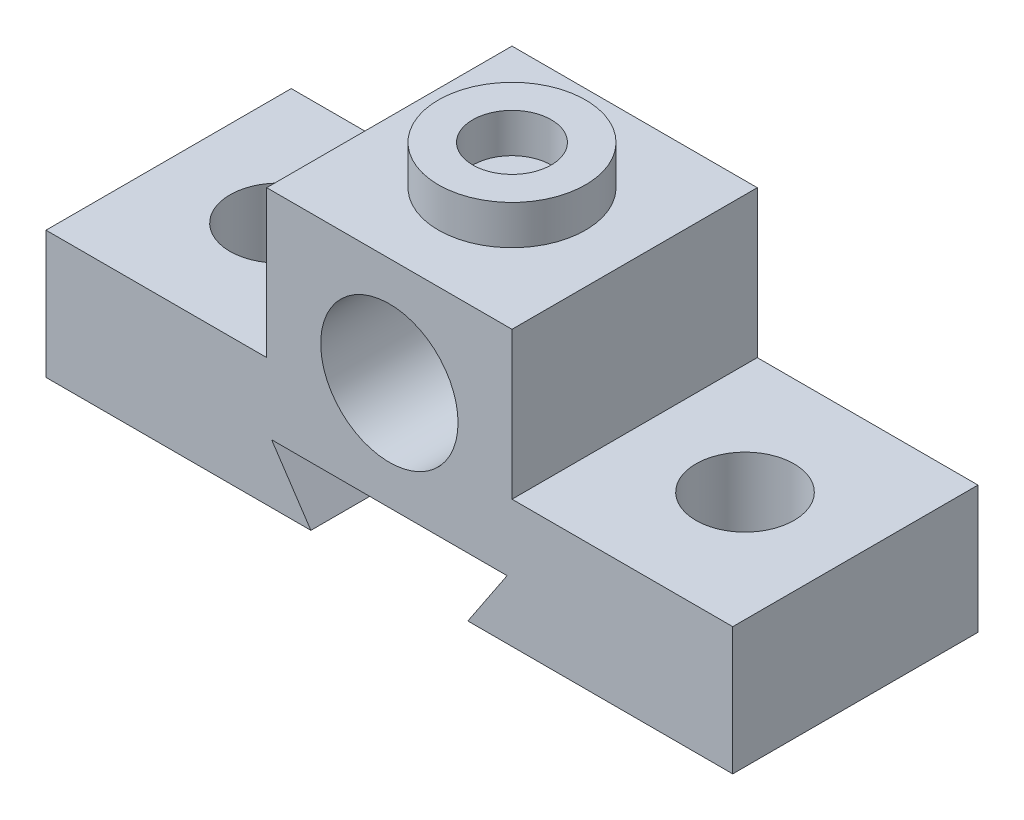
ISO-10303-21;
HEADER;
FILE_DESCRIPTION(('STEP AP214'),'2;1');
FILE_NAME('part.step','',(''),(''),'','','');
FILE_SCHEMA(('AUTOMOTIVE_DESIGN { 1 0 10303 214 1 1 1 1 }'));
ENDSEC;
DATA;
#1=APPLICATION_CONTEXT('core data for automotive mechanical design processes');
#2=APPLICATION_PROTOCOL_DEFINITION('international standard','automotive_design',2000,#1);
#3=PRODUCT_CONTEXT('',#1,'mechanical');
#4=PRODUCT('Part','Part','',(#3));
#5=PRODUCT_RELATED_PRODUCT_CATEGORY('part','',(#4));
#6=PRODUCT_DEFINITION_FORMATION('','',#4);
#7=PRODUCT_DEFINITION_CONTEXT('part definition',#1,'design');
#8=PRODUCT_DEFINITION('design','',#6,#7);
#9=PRODUCT_DEFINITION_SHAPE('','',#8);
#10=(LENGTH_UNIT() NAMED_UNIT(*) SI_UNIT(.MILLI.,.METRE.));
#11=(NAMED_UNIT(*) PLANE_ANGLE_UNIT() SI_UNIT($,.RADIAN.));
#12=(NAMED_UNIT(*) SI_UNIT($,.STERADIAN.) SOLID_ANGLE_UNIT());
#13=UNCERTAINTY_MEASURE_WITH_UNIT(LENGTH_MEASURE(1.E-05),#10,'distance_accuracy_value','');
#14=(GEOMETRIC_REPRESENTATION_CONTEXT(3) GLOBAL_UNCERTAINTY_ASSIGNED_CONTEXT((#13)) GLOBAL_UNIT_ASSIGNED_CONTEXT((#10,
#11,#12)) REPRESENTATION_CONTEXT('',''));
#15=CARTESIAN_POINT('',(0.,0.,0.));
#16=DIRECTION('',(0.,0.,1.));
#17=DIRECTION('',(1.,0.,0.));
#18=AXIS2_PLACEMENT_3D('',#15,#16,#17);
#19=CARTESIAN_POINT('',(0.,0.,25.));
#20=DIRECTION('',(0.,1.,0.));
#21=DIRECTION('',(0.,0.,1.));
#22=AXIS2_PLACEMENT_3D('',#19,#20,#21);
#23=PLANE('',#22);
#24=CARTESIAN_POINT('',(11.25,0.,12.5));
#25=DIRECTION('',(0.,1.,0.));
#26=DIRECTION('',(0.,0.,1.));
#27=AXIS2_PLACEMENT_3D('',#24,#25,#26);
#28=CIRCLE('',#27,5.);
#29=CARTESIAN_POINT('',(11.25,0.,17.5));
#30=VERTEX_POINT('',#29);
#31=EDGE_CURVE('E285',#30,#30,#28,.T.);
#32=ORIENTED_EDGE('',*,*,#31,.T.);
#33=EDGE_LOOP('',(#32));
#34=FACE_BOUND('',#33,.T.);
#35=DIRECTION('',(1.,0.,0.));
#36=VECTOR('',#35,1.);
#37=CARTESIAN_POINT('',(0.,0.,0.));
#38=LINE('',#37,#36);
#39=CARTESIAN_POINT('',(0.,0.,0.));
#40=VERTEX_POINT('',#39);
#41=CARTESIAN_POINT('',(27.,0.,0.));
#42=VERTEX_POINT('',#41);
#43=EDGE_CURVE('E170',#40,#42,#38,.T.);
#44=ORIENTED_EDGE('',*,*,#43,.T.);
#45=DIRECTION('',(0.,0.,-1.));
#46=VECTOR('',#45,1.);
#47=CARTESIAN_POINT('',(27.,0.,25.));
#48=LINE('',#47,#46);
#49=CARTESIAN_POINT('',(27.,0.,25.));
#50=VERTEX_POINT('',#49);
#51=EDGE_CURVE('E48',#50,#42,#48,.T.);
#52=ORIENTED_EDGE('',*,*,#51,.F.);
#53=DIRECTION('',(1.,0.,0.));
#54=VECTOR('',#53,1.);
#55=CARTESIAN_POINT('',(0.,0.,25.));
#56=LINE('',#55,#54);
#57=CARTESIAN_POINT('',(0.,0.,25.));
#58=VERTEX_POINT('',#57);
#59=EDGE_CURVE('E195',#58,#50,#56,.T.);
#60=ORIENTED_EDGE('',*,*,#59,.F.);
#61=DIRECTION('',(0.,0.,-1.));
#62=VECTOR('',#61,1.);
#63=CARTESIAN_POINT('',(0.,0.,25.));
#64=LINE('',#63,#62);
#65=EDGE_CURVE('E162',#58,#40,#64,.T.);
#66=ORIENTED_EDGE('',*,*,#65,.T.);
#67=EDGE_LOOP('',(#44,#52,#60,#66));
#68=FACE_BOUND('',#67,.T.);
#69=ADVANCED_FACE('F44',(#34,#68),#23,.F.);
#70=CARTESIAN_POINT('',(27.,0.,25.));
#71=DIRECTION('',(-0.832050294337844,-0.554700196225229,0.));
#72=DIRECTION('',(0.554700196225229,-0.832050294337844,0.));
#73=AXIS2_PLACEMENT_3D('',#70,#71,#72);
#74=PLANE('',#73);
#75=DIRECTION('',(-0.554700196225229,0.832050294337844,0.));
#76=VECTOR('',#75,1.);
#77=CARTESIAN_POINT('',(27.,0.,0.));
#78=LINE('',#77,#76);
#79=CARTESIAN_POINT('',(23.,6.,0.));
#80=VERTEX_POINT('',#79);
#81=EDGE_CURVE('E168',#42,#80,#78,.T.);
#82=ORIENTED_EDGE('',*,*,#81,.T.);
#83=DIRECTION('',(0.,0.,-1.));
#84=VECTOR('',#83,1.);
#85=CARTESIAN_POINT('',(23.,6.,25.));
#86=LINE('',#85,#84);
#87=CARTESIAN_POINT('',(23.,6.,25.));
#88=VERTEX_POINT('',#87);
#89=EDGE_CURVE('E213',#88,#80,#86,.T.);
#90=ORIENTED_EDGE('',*,*,#89,.F.);
#91=DIRECTION('',(-0.554700196225229,0.832050294337844,0.));
#92=VECTOR('',#91,1.);
#93=CARTESIAN_POINT('',(27.,0.,25.));
#94=LINE('',#93,#92);
#95=EDGE_CURVE('E120',#50,#88,#94,.T.);
#96=ORIENTED_EDGE('',*,*,#95,.F.);
#97=ORIENTED_EDGE('',*,*,#51,.T.);
#98=EDGE_LOOP('',(#82,#90,#96,#97));
#99=FACE_BOUND('',#98,.T.);
#100=ADVANCED_FACE('F217',(#99),#74,.F.);
#101=CARTESIAN_POINT('',(35.,6.,25.));
#102=DIRECTION('',(0.,1.,0.));
#103=DIRECTION('',(0.,0.,1.));
#104=AXIS2_PLACEMENT_3D('',#101,#102,#103);
#105=PLANE('',#104);
#106=DIRECTION('',(1.,0.,0.));
#107=VECTOR('',#106,1.);
#108=CARTESIAN_POINT('',(35.,6.,0.));
#109=LINE('',#108,#107);
#110=CARTESIAN_POINT('',(47.,6.,0.));
#111=VERTEX_POINT('',#110);
#112=EDGE_CURVE('E171',#80,#111,#109,.T.);
#113=ORIENTED_EDGE('',*,*,#112,.T.);
#114=DIRECTION('',(0.,0.,-1.));
#115=VECTOR('',#114,1.);
#116=CARTESIAN_POINT('',(47.,6.,25.));
#117=LINE('',#116,#115);
#118=CARTESIAN_POINT('',(47.,6.,25.));
#119=VERTEX_POINT('',#118);
#120=EDGE_CURVE('E211',#119,#111,#117,.T.);
#121=ORIENTED_EDGE('',*,*,#120,.F.);
#122=DIRECTION('',(1.,0.,0.));
#123=VECTOR('',#122,1.);
#124=CARTESIAN_POINT('',(35.,6.,25.));
#125=LINE('',#124,#123);
#126=EDGE_CURVE('E232',#88,#119,#125,.T.);
#127=ORIENTED_EDGE('',*,*,#126,.F.);
#128=ORIENTED_EDGE('',*,*,#89,.T.);
#129=EDGE_LOOP('',(#113,#121,#127,#128));
#130=FACE_BOUND('',#129,.T.);
#131=ADVANCED_FACE('F229',(#130),#105,.F.);
#132=CARTESIAN_POINT('',(43.,0.,25.));
#133=DIRECTION('',(0.832050294337844,-0.554700196225228,0.));
#134=DIRECTION('',(0.554700196225228,0.832050294337844,0.));
#135=AXIS2_PLACEMENT_3D('',#132,#133,#134);
#136=PLANE('',#135);
#137=DIRECTION('',(-0.554700196225228,-0.832050294337844,0.));
#138=VECTOR('',#137,1.);
#139=CARTESIAN_POINT('',(43.,0.,0.));
#140=LINE('',#139,#138);
#141=CARTESIAN_POINT('',(43.,0.,0.));
#142=VERTEX_POINT('',#141);
#143=EDGE_CURVE('E178',#111,#142,#140,.T.);
#144=ORIENTED_EDGE('',*,*,#143,.T.);
#145=DIRECTION('',(0.,0.,-1.));
#146=VECTOR('',#145,1.);
#147=CARTESIAN_POINT('',(43.,0.,25.));
#148=LINE('',#147,#146);
#149=CARTESIAN_POINT('',(43.,0.,25.));
#150=VERTEX_POINT('',#149);
#151=EDGE_CURVE('E208',#150,#142,#148,.T.);
#152=ORIENTED_EDGE('',*,*,#151,.F.);
#153=DIRECTION('',(-0.554700196225228,-0.832050294337844,0.));
#154=VECTOR('',#153,1.);
#155=CARTESIAN_POINT('',(43.,0.,25.));
#156=LINE('',#155,#154);
#157=EDGE_CURVE('E235',#119,#150,#156,.T.);
#158=ORIENTED_EDGE('',*,*,#157,.F.);
#159=ORIENTED_EDGE('',*,*,#120,.T.);
#160=EDGE_LOOP('',(#144,#152,#158,#159));
#161=FACE_BOUND('',#160,.T.);
#162=ADVANCED_FACE('F228',(#161),#136,.F.);
#163=CARTESIAN_POINT('',(70.,0.,25.));
#164=DIRECTION('',(0.,1.,0.));
#165=DIRECTION('',(0.,0.,1.));
#166=AXIS2_PLACEMENT_3D('',#163,#164,#165);
#167=PLANE('',#166);
#168=CARTESIAN_POINT('',(58.75,0.,12.5));
#169=DIRECTION('',(0.,1.,0.));
#170=DIRECTION('',(0.,0.,1.));
#171=AXIS2_PLACEMENT_3D('',#168,#169,#170);
#172=CIRCLE('',#171,5.);
#173=CARTESIAN_POINT('',(58.75,0.,17.5));
#174=VERTEX_POINT('',#173);
#175=EDGE_CURVE('E289',#174,#174,#172,.T.);
#176=ORIENTED_EDGE('',*,*,#175,.T.);
#177=EDGE_LOOP('',(#176));
#178=FACE_BOUND('',#177,.T.);
#179=DIRECTION('',(1.,0.,0.));
#180=VECTOR('',#179,1.);
#181=CARTESIAN_POINT('',(70.,0.,0.));
#182=LINE('',#181,#180);
#183=CARTESIAN_POINT('',(70.,0.,0.));
#184=VERTEX_POINT('',#183);
#185=EDGE_CURVE('E176',#142,#184,#182,.T.);
#186=ORIENTED_EDGE('',*,*,#185,.T.);
#187=DIRECTION('',(0.,0.,-1.));
#188=VECTOR('',#187,1.);
#189=CARTESIAN_POINT('',(70.,0.,25.));
#190=LINE('',#189,#188);
#191=CARTESIAN_POINT('',(70.,0.,25.));
#192=VERTEX_POINT('',#191);
#193=EDGE_CURVE('E202',#192,#184,#190,.T.);
#194=ORIENTED_EDGE('',*,*,#193,.F.);
#195=DIRECTION('',(1.,0.,0.));
#196=VECTOR('',#195,1.);
#197=CARTESIAN_POINT('',(70.,0.,25.));
#198=LINE('',#197,#196);
#199=EDGE_CURVE('E234',#150,#192,#198,.T.);
#200=ORIENTED_EDGE('',*,*,#199,.F.);
#201=ORIENTED_EDGE('',*,*,#151,.T.);
#202=EDGE_LOOP('',(#186,#194,#200,#201));
#203=FACE_BOUND('',#202,.T.);
#204=ADVANCED_FACE('F264',(#178,#203),#167,.F.);
#205=CARTESIAN_POINT('',(70.,0.,25.));
#206=DIRECTION('',(-1.,0.,0.));
#207=DIRECTION('',(0.,0.,1.));
#208=AXIS2_PLACEMENT_3D('',#205,#206,#207);
#209=PLANE('',#208);
#210=DIRECTION('',(0.,1.,0.));
#211=VECTOR('',#210,1.);
#212=CARTESIAN_POINT('',(70.,0.,0.));
#213=LINE('',#212,#211);
#214=CARTESIAN_POINT('',(70.,13.,0.));
#215=VERTEX_POINT('',#214);
#216=EDGE_CURVE('E177',#184,#215,#213,.T.);
#217=ORIENTED_EDGE('',*,*,#216,.T.);
#218=DIRECTION('',(0.,0.,-1.));
#219=VECTOR('',#218,1.);
#220=CARTESIAN_POINT('',(70.,13.,25.));
#221=LINE('',#220,#219);
#222=CARTESIAN_POINT('',(70.,13.,25.));
#223=VERTEX_POINT('',#222);
#224=EDGE_CURVE('E205',#223,#215,#221,.T.);
#225=ORIENTED_EDGE('',*,*,#224,.F.);
#226=DIRECTION('',(0.,1.,0.));
#227=VECTOR('',#226,1.);
#228=CARTESIAN_POINT('',(70.,0.,25.));
#229=LINE('',#228,#227);
#230=EDGE_CURVE('E240',#192,#223,#229,.T.);
#231=ORIENTED_EDGE('',*,*,#230,.F.);
#232=ORIENTED_EDGE('',*,*,#193,.T.);
#233=EDGE_LOOP('',(#217,#225,#231,#232));
#234=FACE_BOUND('',#233,.T.);
#235=ADVANCED_FACE('F265',(#234),#209,.F.);
#236=CARTESIAN_POINT('',(47.5,13.,25.));
#237=DIRECTION('',(0.,-1.,0.));
#238=DIRECTION('',(0.,0.,-1.));
#239=AXIS2_PLACEMENT_3D('',#236,#237,#238);
#240=PLANE('',#239);
#241=CARTESIAN_POINT('',(58.75,13.,12.5));
#242=DIRECTION('',(0.,1.,0.));
#243=DIRECTION('',(0.,0.,1.));
#244=AXIS2_PLACEMENT_3D('',#241,#242,#243);
#245=CIRCLE('',#244,5.);
#246=CARTESIAN_POINT('',(58.75,13.,17.5));
#247=VERTEX_POINT('',#246);
#248=EDGE_CURVE('E283',#247,#247,#245,.T.);
#249=ORIENTED_EDGE('',*,*,#248,.F.);
#250=EDGE_LOOP('',(#249));
#251=FACE_BOUND('',#250,.T.);
#252=DIRECTION('',(-1.,0.,0.));
#253=VECTOR('',#252,1.);
#254=CARTESIAN_POINT('',(47.5,13.,0.));
#255=LINE('',#254,#253);
#256=CARTESIAN_POINT('',(47.5,13.,0.));
#257=VERTEX_POINT('',#256);
#258=EDGE_CURVE('E185',#215,#257,#255,.T.);
#259=ORIENTED_EDGE('',*,*,#258,.T.);
#260=DIRECTION('',(0.,0.,-1.));
#261=VECTOR('',#260,1.);
#262=CARTESIAN_POINT('',(47.5,13.,25.));
#263=LINE('',#262,#261);
#264=CARTESIAN_POINT('',(47.5,13.,25.));
#265=VERTEX_POINT('',#264);
#266=EDGE_CURVE('E200',#265,#257,#263,.T.);
#267=ORIENTED_EDGE('',*,*,#266,.F.);
#268=DIRECTION('',(-1.,0.,0.));
#269=VECTOR('',#268,1.);
#270=CARTESIAN_POINT('',(47.5,13.,25.));
#271=LINE('',#270,#269);
#272=EDGE_CURVE('E245',#223,#265,#271,.T.);
#273=ORIENTED_EDGE('',*,*,#272,.F.);
#274=ORIENTED_EDGE('',*,*,#224,.T.);
#275=EDGE_LOOP('',(#259,#267,#273,#274));
#276=FACE_BOUND('',#275,.T.);
#277=ADVANCED_FACE('F256',(#251,#276),#240,.F.);
#278=CARTESIAN_POINT('',(47.5,28.,25.));
#279=DIRECTION('',(-1.,0.,0.));
#280=DIRECTION('',(0.,0.,1.));
#281=AXIS2_PLACEMENT_3D('',#278,#279,#280);
#282=PLANE('',#281);
#283=DIRECTION('',(0.,1.,0.));
#284=VECTOR('',#283,1.);
#285=CARTESIAN_POINT('',(47.5,28.,0.));
#286=LINE('',#285,#284);
#287=CARTESIAN_POINT('',(47.5,28.,0.));
#288=VERTEX_POINT('',#287);
#289=EDGE_CURVE('E184',#257,#288,#286,.T.);
#290=ORIENTED_EDGE('',*,*,#289,.T.);
#291=DIRECTION('',(0.,0.,-1.));
#292=VECTOR('',#291,1.);
#293=CARTESIAN_POINT('',(47.5,28.,25.));
#294=LINE('',#293,#292);
#295=CARTESIAN_POINT('',(47.5,28.,25.));
#296=VERTEX_POINT('',#295);
#297=EDGE_CURVE('E198',#296,#288,#294,.T.);
#298=ORIENTED_EDGE('',*,*,#297,.F.);
#299=DIRECTION('',(0.,1.,0.));
#300=VECTOR('',#299,1.);
#301=CARTESIAN_POINT('',(47.5,28.,25.));
#302=LINE('',#301,#300);
#303=EDGE_CURVE('E243',#265,#296,#302,.T.);
#304=ORIENTED_EDGE('',*,*,#303,.F.);
#305=ORIENTED_EDGE('',*,*,#266,.T.);
#306=EDGE_LOOP('',(#290,#298,#304,#305));
#307=FACE_BOUND('',#306,.T.);
#308=ADVANCED_FACE('F253',(#307),#282,.F.);
#309=CARTESIAN_POINT('',(35.,28.,25.));
#310=DIRECTION('',(0.,-1.,0.));
#311=DIRECTION('',(0.,0.,-1.));
#312=AXIS2_PLACEMENT_3D('',#309,#310,#311);
#313=PLANE('',#312);
#314=CARTESIAN_POINT('',(35.,28.,12.5));
#315=DIRECTION('',(0.,1.,0.));
#316=DIRECTION('',(0.,0.,1.));
#317=AXIS2_PLACEMENT_3D('',#314,#315,#316);
#318=CIRCLE('',#317,7.5);
#319=CARTESIAN_POINT('',(35.,28.,20.));
#320=VERTEX_POINT('',#319);
#321=EDGE_CURVE('E11',#320,#320,#318,.T.);
#322=ORIENTED_EDGE('',*,*,#321,.F.);
#323=EDGE_LOOP('',(#322));
#324=FACE_BOUND('',#323,.T.);
#325=DIRECTION('',(-1.,0.,0.));
#326=VECTOR('',#325,1.);
#327=CARTESIAN_POINT('',(35.,28.,0.));
#328=LINE('',#327,#326);
#329=CARTESIAN_POINT('',(22.5,28.,0.));
#330=VERTEX_POINT('',#329);
#331=EDGE_CURVE('E189',#288,#330,#328,.T.);
#332=ORIENTED_EDGE('',*,*,#331,.T.);
#333=DIRECTION('',(0.,0.,-1.));
#334=VECTOR('',#333,1.);
#335=CARTESIAN_POINT('',(22.5,28.,25.));
#336=LINE('',#335,#334);
#337=CARTESIAN_POINT('',(22.5,28.,25.));
#338=VERTEX_POINT('',#337);
#339=EDGE_CURVE('E158',#338,#330,#336,.T.);
#340=ORIENTED_EDGE('',*,*,#339,.F.);
#341=DIRECTION('',(-1.,0.,0.));
#342=VECTOR('',#341,1.);
#343=CARTESIAN_POINT('',(35.,28.,25.));
#344=LINE('',#343,#342);
#345=EDGE_CURVE('E149',#296,#338,#344,.T.);
#346=ORIENTED_EDGE('',*,*,#345,.F.);
#347=ORIENTED_EDGE('',*,*,#297,.T.);
#348=EDGE_LOOP('',(#332,#340,#346,#347));
#349=FACE_BOUND('',#348,.T.);
#350=ADVANCED_FACE('F255',(#324,#349),#313,.F.);
#351=CARTESIAN_POINT('',(22.5,28.,25.));
#352=DIRECTION('',(1.,0.,0.));
#353=DIRECTION('',(0.,0.,-1.));
#354=AXIS2_PLACEMENT_3D('',#351,#352,#353);
#355=PLANE('',#354);
#356=DIRECTION('',(0.,-1.,0.));
#357=VECTOR('',#356,1.);
#358=CARTESIAN_POINT('',(22.5,28.,0.));
#359=LINE('',#358,#357);
#360=CARTESIAN_POINT('',(22.5,13.,0.));
#361=VERTEX_POINT('',#360);
#362=EDGE_CURVE('E160',#330,#361,#359,.T.);
#363=ORIENTED_EDGE('',*,*,#362,.T.);
#364=DIRECTION('',(0.,0.,-1.));
#365=VECTOR('',#364,1.);
#366=CARTESIAN_POINT('',(22.5,13.,25.));
#367=LINE('',#366,#365);
#368=CARTESIAN_POINT('',(22.5,13.,25.));
#369=VERTEX_POINT('',#368);
#370=EDGE_CURVE('E152',#369,#361,#367,.T.);
#371=ORIENTED_EDGE('',*,*,#370,.F.);
#372=DIRECTION('',(0.,-1.,0.));
#373=VECTOR('',#372,1.);
#374=CARTESIAN_POINT('',(22.5,28.,25.));
#375=LINE('',#374,#373);
#376=EDGE_CURVE('E141',#338,#369,#375,.T.);
#377=ORIENTED_EDGE('',*,*,#376,.F.);
#378=ORIENTED_EDGE('',*,*,#339,.T.);
#379=EDGE_LOOP('',(#363,#371,#377,#378));
#380=FACE_BOUND('',#379,.T.);
#381=ADVANCED_FACE('F154',(#380),#355,.F.);
#382=CARTESIAN_POINT('',(22.5,13.,25.));
#383=DIRECTION('',(0.,-1.,0.));
#384=DIRECTION('',(0.,0.,-1.));
#385=AXIS2_PLACEMENT_3D('',#382,#383,#384);
#386=PLANE('',#385);
#387=CARTESIAN_POINT('',(11.25,13.,12.5));
#388=DIRECTION('',(0.,1.,0.));
#389=DIRECTION('',(0.,0.,1.));
#390=AXIS2_PLACEMENT_3D('',#387,#388,#389);
#391=CIRCLE('',#390,5.);
#392=CARTESIAN_POINT('',(11.25,13.,17.5));
#393=VERTEX_POINT('',#392);
#394=EDGE_CURVE('E288',#393,#393,#391,.T.);
#395=ORIENTED_EDGE('',*,*,#394,.F.);
#396=EDGE_LOOP('',(#395));
#397=FACE_BOUND('',#396,.T.);
#398=DIRECTION('',(-1.,0.,0.));
#399=VECTOR('',#398,1.);
#400=CARTESIAN_POINT('',(22.5,13.,0.));
#401=LINE('',#400,#399);
#402=CARTESIAN_POINT('',(0.,13.,0.));
#403=VERTEX_POINT('',#402);
#404=EDGE_CURVE('E103',#361,#403,#401,.T.);
#405=ORIENTED_EDGE('',*,*,#404,.T.);
#406=DIRECTION('',(0.,0.,-1.));
#407=VECTOR('',#406,1.);
#408=CARTESIAN_POINT('',(0.,13.,25.));
#409=LINE('',#408,#407);
#410=CARTESIAN_POINT('',(0.,13.,25.));
#411=VERTEX_POINT('',#410);
#412=EDGE_CURVE('E157',#411,#403,#409,.T.);
#413=ORIENTED_EDGE('',*,*,#412,.F.);
#414=DIRECTION('',(-1.,0.,0.));
#415=VECTOR('',#414,1.);
#416=CARTESIAN_POINT('',(22.5,13.,25.));
#417=LINE('',#416,#415);
#418=EDGE_CURVE('E150',#369,#411,#417,.T.);
#419=ORIENTED_EDGE('',*,*,#418,.F.);
#420=ORIENTED_EDGE('',*,*,#370,.T.);
#421=EDGE_LOOP('',(#405,#413,#419,#420));
#422=FACE_BOUND('',#421,.T.);
#423=ADVANCED_FACE('F161',(#397,#422),#386,.F.);
#424=CARTESIAN_POINT('',(0.,0.,25.));
#425=DIRECTION('',(1.,0.,0.));
#426=DIRECTION('',(0.,0.,-1.));
#427=AXIS2_PLACEMENT_3D('',#424,#425,#426);
#428=PLANE('',#427);
#429=DIRECTION('',(0.,-1.,0.));
#430=VECTOR('',#429,1.);
#431=CARTESIAN_POINT('',(0.,0.,0.));
#432=LINE('',#431,#430);
#433=EDGE_CURVE('E108',#403,#40,#432,.T.);
#434=ORIENTED_EDGE('',*,*,#433,.T.);
#435=ORIENTED_EDGE('',*,*,#65,.F.);
#436=DIRECTION('',(0.,-1.,0.));
#437=VECTOR('',#436,1.);
#438=CARTESIAN_POINT('',(0.,0.,25.));
#439=LINE('',#438,#437);
#440=EDGE_CURVE('E64',#411,#58,#439,.T.);
#441=ORIENTED_EDGE('',*,*,#440,.F.);
#442=ORIENTED_EDGE('',*,*,#412,.T.);
#443=EDGE_LOOP('',(#434,#435,#441,#442));
#444=FACE_BOUND('',#443,.T.);
#445=ADVANCED_FACE('F368',(#444),#428,.F.);
#446=CARTESIAN_POINT('',(0.,0.,25.));
#447=DIRECTION('',(0.,0.,1.));
#448=DIRECTION('',(1.,0.,0.));
#449=AXIS2_PLACEMENT_3D('',#446,#447,#448);
#450=PLANE('',#449);
#451=CARTESIAN_POINT('',(35.,17.,25.));
#452=DIRECTION('',(0.,0.,1.));
#453=DIRECTION('',(1.,0.,0.));
#454=AXIS2_PLACEMENT_3D('',#451,#452,#453);
#455=CIRCLE('',#454,7.);
#456=CARTESIAN_POINT('',(42.,17.,25.));
#457=VERTEX_POINT('',#456);
#458=EDGE_CURVE('E300',#457,#457,#455,.T.);
#459=ORIENTED_EDGE('',*,*,#458,.F.);
#460=EDGE_LOOP('',(#459));
#461=FACE_BOUND('',#460,.T.);
#462=ORIENTED_EDGE('',*,*,#59,.T.);
#463=ORIENTED_EDGE('',*,*,#95,.T.);
#464=ORIENTED_EDGE('',*,*,#126,.T.);
#465=ORIENTED_EDGE('',*,*,#157,.T.);
#466=ORIENTED_EDGE('',*,*,#199,.T.);
#467=ORIENTED_EDGE('',*,*,#230,.T.);
#468=ORIENTED_EDGE('',*,*,#272,.T.);
#469=ORIENTED_EDGE('',*,*,#303,.T.);
#470=ORIENTED_EDGE('',*,*,#345,.T.);
#471=ORIENTED_EDGE('',*,*,#376,.T.);
#472=ORIENTED_EDGE('',*,*,#418,.T.);
#473=ORIENTED_EDGE('',*,*,#440,.T.);
#474=EDGE_LOOP('',(#462,#463,#464,#465,#466,#467,#468,#469,#470,#471,#472,#473));
#475=FACE_BOUND('',#474,.T.);
#476=ADVANCED_FACE('F144',(#461,#475),#450,.T.);
#477=CARTESIAN_POINT('',(0.,0.,0.));
#478=DIRECTION('',(0.,0.,1.));
#479=DIRECTION('',(1.,0.,0.));
#480=AXIS2_PLACEMENT_3D('',#477,#478,#479);
#481=PLANE('',#480);
#482=CARTESIAN_POINT('',(35.,17.,0.));
#483=DIRECTION('',(0.,0.,1.));
#484=DIRECTION('',(1.,0.,0.));
#485=AXIS2_PLACEMENT_3D('',#482,#483,#484);
#486=CIRCLE('',#485,7.);
#487=CARTESIAN_POINT('',(42.,17.,0.));
#488=VERTEX_POINT('',#487);
#489=EDGE_CURVE('E172',#488,#488,#486,.T.);
#490=ORIENTED_EDGE('',*,*,#489,.T.);
#491=EDGE_LOOP('',(#490));
#492=FACE_BOUND('',#491,.T.);
#493=ORIENTED_EDGE('',*,*,#43,.F.);
#494=ORIENTED_EDGE('',*,*,#433,.F.);
#495=ORIENTED_EDGE('',*,*,#404,.F.);
#496=ORIENTED_EDGE('',*,*,#362,.F.);
#497=ORIENTED_EDGE('',*,*,#331,.F.);
#498=ORIENTED_EDGE('',*,*,#289,.F.);
#499=ORIENTED_EDGE('',*,*,#258,.F.);
#500=ORIENTED_EDGE('',*,*,#216,.F.);
#501=ORIENTED_EDGE('',*,*,#185,.F.);
#502=ORIENTED_EDGE('',*,*,#143,.F.);
#503=ORIENTED_EDGE('',*,*,#112,.F.);
#504=ORIENTED_EDGE('',*,*,#81,.F.);
#505=EDGE_LOOP('',(#493,#494,#495,#496,#497,#498,#499,#500,#501,#502,#503,#504));
#506=FACE_BOUND('',#505,.T.);
#507=ADVANCED_FACE('F224',(#492,#506),#481,.F.);
#508=CARTESIAN_POINT('',(35.,17.,0.));
#509=DIRECTION('',(0.,0.,1.));
#510=DIRECTION('',(1.,0.,0.));
#511=AXIS2_PLACEMENT_3D('',#508,#509,#510);
#512=CYLINDRICAL_SURFACE('',#511,7.);
#513=ORIENTED_EDGE('',*,*,#489,.F.);
#514=EDGE_LOOP('',(#513));
#515=FACE_BOUND('',#514,.T.);
#516=ORIENTED_EDGE('',*,*,#458,.T.);
#517=EDGE_LOOP('',(#516));
#518=FACE_BOUND('',#517,.T.);
#519=ADVANCED_FACE('F356',(#515,#518),#512,.F.);
#520=CARTESIAN_POINT('',(11.25,0.,12.5));
#521=DIRECTION('',(0.,1.,0.));
#522=DIRECTION('',(0.,0.,1.));
#523=AXIS2_PLACEMENT_3D('',#520,#521,#522);
#524=CYLINDRICAL_SURFACE('',#523,5.);
#525=CARTESIAN_POINT('',(11.25,0.,17.5));
#526=CARTESIAN_POINT('',(11.25,0.135416666666666,17.5));
#527=CARTESIAN_POINT('',(11.25,0.270833333333333,17.5));
#528=CARTESIAN_POINT('',(11.25,0.541666666666667,17.5));
#529=CARTESIAN_POINT('',(11.25,0.677083333333333,17.5));
#530=CARTESIAN_POINT('',(11.25,0.947916666666667,17.5));
#531=CARTESIAN_POINT('',(11.25,1.08333333333333,17.5));
#532=CARTESIAN_POINT('',(11.25,1.35416666666667,17.5));
#533=CARTESIAN_POINT('',(11.25,1.48958333333333,17.5));
#534=CARTESIAN_POINT('',(11.25,1.76041666666667,17.5));
#535=CARTESIAN_POINT('',(11.25,1.89583333333333,17.5));
#536=CARTESIAN_POINT('',(11.25,2.16666666666667,17.5));
#537=CARTESIAN_POINT('',(11.25,2.30208333333333,17.5));
#538=CARTESIAN_POINT('',(11.25,2.57291666666667,17.5));
#539=CARTESIAN_POINT('',(11.25,2.70833333333333,17.5));
#540=CARTESIAN_POINT('',(11.25,2.97916666666667,17.5));
#541=CARTESIAN_POINT('',(11.25,3.11458333333333,17.5));
#542=CARTESIAN_POINT('',(11.25,3.38541666666667,17.5));
#543=CARTESIAN_POINT('',(11.25,3.52083333333333,17.5));
#544=CARTESIAN_POINT('',(11.25,3.79166666666667,17.5));
#545=CARTESIAN_POINT('',(11.25,3.92708333333333,17.5));
#546=CARTESIAN_POINT('',(11.25,4.19791666666667,17.5));
#547=CARTESIAN_POINT('',(11.25,4.33333333333333,17.5));
#548=CARTESIAN_POINT('',(11.25,4.60416666666667,17.5));
#549=CARTESIAN_POINT('',(11.25,4.73958333333333,17.5));
#550=CARTESIAN_POINT('',(11.25,5.01041666666667,17.5));
#551=CARTESIAN_POINT('',(11.25,5.14583333333333,17.5));
#552=CARTESIAN_POINT('',(11.25,5.41666666666667,17.5));
#553=CARTESIAN_POINT('',(11.25,5.55208333333333,17.5));
#554=CARTESIAN_POINT('',(11.25,5.82291666666667,17.5));
#555=CARTESIAN_POINT('',(11.25,5.95833333333333,17.5));
#556=CARTESIAN_POINT('',(11.25,6.22916666666667,17.5));
#557=CARTESIAN_POINT('',(11.25,6.36458333333333,17.5));
#558=CARTESIAN_POINT('',(11.25,6.63541666666667,17.5));
#559=CARTESIAN_POINT('',(11.25,6.77083333333333,17.5));
#560=CARTESIAN_POINT('',(11.25,7.04166666666667,17.5));
#561=CARTESIAN_POINT('',(11.25,7.17708333333333,17.5));
#562=CARTESIAN_POINT('',(11.25,7.44791666666667,17.5));
#563=CARTESIAN_POINT('',(11.25,7.58333333333333,17.5));
#564=CARTESIAN_POINT('',(11.25,7.85416666666667,17.5));
#565=CARTESIAN_POINT('',(11.25,7.98958333333333,17.5));
#566=CARTESIAN_POINT('',(11.25,8.26041666666667,17.5));
#567=CARTESIAN_POINT('',(11.25,8.39583333333333,17.5));
#568=CARTESIAN_POINT('',(11.25,8.66666666666667,17.5));
#569=CARTESIAN_POINT('',(11.25,8.80208333333333,17.5));
#570=CARTESIAN_POINT('',(11.25,9.07291666666667,17.5));
#571=CARTESIAN_POINT('',(11.25,9.20833333333333,17.5));
#572=CARTESIAN_POINT('',(11.25,9.47916666666667,17.5));
#573=CARTESIAN_POINT('',(11.25,9.61458333333333,17.5));
#574=CARTESIAN_POINT('',(11.25,9.88541666666667,17.5));
#575=CARTESIAN_POINT('',(11.25,10.0208333333333,17.5));
#576=CARTESIAN_POINT('',(11.25,10.2916666666667,17.5));
#577=CARTESIAN_POINT('',(11.25,10.4270833333333,17.5));
#578=CARTESIAN_POINT('',(11.25,10.6979166666667,17.5));
#579=CARTESIAN_POINT('',(11.25,10.8333333333333,17.5));
#580=CARTESIAN_POINT('',(11.25,11.1041666666667,17.5));
#581=CARTESIAN_POINT('',(11.25,11.2395833333333,17.5));
#582=CARTESIAN_POINT('',(11.25,11.5104166666667,17.5));
#583=CARTESIAN_POINT('',(11.25,11.6458333333333,17.5));
#584=CARTESIAN_POINT('',(11.25,11.9166666666667,17.5));
#585=CARTESIAN_POINT('',(11.25,12.0520833333333,17.5));
#586=CARTESIAN_POINT('',(11.25,12.3229166666667,17.5));
#587=CARTESIAN_POINT('',(11.25,12.4583333333333,17.5));
#588=CARTESIAN_POINT('',(11.25,12.7291666666667,17.5));
#589=CARTESIAN_POINT('',(11.25,12.8645833333333,17.5));
#590=CARTESIAN_POINT('',(11.25,13.,17.5));
#591=B_SPLINE_CURVE_WITH_KNOTS('',3,(#525,#526,#527,#528,#529,#530,#531,#532,#533,#534,#535,
#536,#537,#538,#539,#540,#541,#542,#543,#544,#545,#546,#547,#548,#549,#550,#551,#552,#553,#554,
#555,#556,#557,#558,#559,#560,#561,#562,#563,#564,#565,#566,#567,#568,#569,#570,#571,#572,#573,
#574,#575,#576,#577,#578,#579,#580,#581,#582,#583,#584,#585,#586,#587,#588,#589,#590),
.UNSPECIFIED.,.F.,.F.,(4,2,2,2,2,2,2,2,2,2,2,2,2,2,2,2,2,2,2,2,2,2,2,2,2,2,2,2,2,2,2,2,4),(0.,
0.40625,0.8125,1.21875,1.625,2.03125,2.4375,2.84375,3.25,3.65625,4.0625,4.46875,4.875,5.28125,
5.6875,6.09375,6.5,6.90625,7.3125,7.71875,8.125,8.53125,8.9375,9.34375,9.75,10.15625,10.5625,
10.96875,11.375,11.78125,12.1875,12.59375,13.),.UNSPECIFIED.);
#592=EDGE_CURVE('BSEAM354',#30,#393,#591,.T.);
#593=ORIENTED_EDGE('',*,*,#31,.F.);
#594=ORIENTED_EDGE('',*,*,#394,.T.);
#595=ORIENTED_EDGE('',*,*,#592,.T.);
#596=ORIENTED_EDGE('',*,*,#592,.F.);
#597=EDGE_LOOP('',(#593,#595,#594,#596));
#598=FACE_BOUND('',#597,.T.);
#599=ADVANCED_FACE('F354',(#598),#524,.F.);
#600=CARTESIAN_POINT('',(58.75,0.,12.5));
#601=DIRECTION('',(0.,1.,0.));
#602=DIRECTION('',(0.,0.,1.));
#603=AXIS2_PLACEMENT_3D('',#600,#601,#602);
#604=CYLINDRICAL_SURFACE('',#603,5.);
#605=CARTESIAN_POINT('',(58.75,0.,17.5));
#606=CARTESIAN_POINT('',(58.75,0.135416666666666,17.5));
#607=CARTESIAN_POINT('',(58.75,0.270833333333333,17.5));
#608=CARTESIAN_POINT('',(58.75,0.541666666666667,17.5));
#609=CARTESIAN_POINT('',(58.75,0.677083333333333,17.5));
#610=CARTESIAN_POINT('',(58.75,0.947916666666667,17.5));
#611=CARTESIAN_POINT('',(58.75,1.08333333333333,17.5));
#612=CARTESIAN_POINT('',(58.75,1.35416666666667,17.5));
#613=CARTESIAN_POINT('',(58.75,1.48958333333333,17.5));
#614=CARTESIAN_POINT('',(58.75,1.76041666666667,17.5));
#615=CARTESIAN_POINT('',(58.75,1.89583333333333,17.5));
#616=CARTESIAN_POINT('',(58.75,2.16666666666667,17.5));
#617=CARTESIAN_POINT('',(58.75,2.30208333333333,17.5));
#618=CARTESIAN_POINT('',(58.75,2.57291666666667,17.5));
#619=CARTESIAN_POINT('',(58.75,2.70833333333333,17.5));
#620=CARTESIAN_POINT('',(58.75,2.97916666666667,17.5));
#621=CARTESIAN_POINT('',(58.75,3.11458333333333,17.5));
#622=CARTESIAN_POINT('',(58.75,3.38541666666667,17.5));
#623=CARTESIAN_POINT('',(58.75,3.52083333333333,17.5));
#624=CARTESIAN_POINT('',(58.75,3.79166666666667,17.5));
#625=CARTESIAN_POINT('',(58.75,3.92708333333333,17.5));
#626=CARTESIAN_POINT('',(58.75,4.19791666666667,17.5));
#627=CARTESIAN_POINT('',(58.75,4.33333333333333,17.5));
#628=CARTESIAN_POINT('',(58.75,4.60416666666667,17.5));
#629=CARTESIAN_POINT('',(58.75,4.73958333333333,17.5));
#630=CARTESIAN_POINT('',(58.75,5.01041666666667,17.5));
#631=CARTESIAN_POINT('',(58.75,5.14583333333333,17.5));
#632=CARTESIAN_POINT('',(58.75,5.41666666666667,17.5));
#633=CARTESIAN_POINT('',(58.75,5.55208333333333,17.5));
#634=CARTESIAN_POINT('',(58.75,5.82291666666667,17.5));
#635=CARTESIAN_POINT('',(58.75,5.95833333333333,17.5));
#636=CARTESIAN_POINT('',(58.75,6.22916666666667,17.5));
#637=CARTESIAN_POINT('',(58.75,6.36458333333333,17.5));
#638=CARTESIAN_POINT('',(58.75,6.63541666666667,17.5));
#639=CARTESIAN_POINT('',(58.75,6.77083333333333,17.5));
#640=CARTESIAN_POINT('',(58.75,7.04166666666667,17.5));
#641=CARTESIAN_POINT('',(58.75,7.17708333333333,17.5));
#642=CARTESIAN_POINT('',(58.75,7.44791666666667,17.5));
#643=CARTESIAN_POINT('',(58.75,7.58333333333333,17.5));
#644=CARTESIAN_POINT('',(58.75,7.85416666666667,17.5));
#645=CARTESIAN_POINT('',(58.75,7.98958333333333,17.5));
#646=CARTESIAN_POINT('',(58.75,8.26041666666667,17.5));
#647=CARTESIAN_POINT('',(58.75,8.39583333333333,17.5));
#648=CARTESIAN_POINT('',(58.75,8.66666666666667,17.5));
#649=CARTESIAN_POINT('',(58.75,8.80208333333333,17.5));
#650=CARTESIAN_POINT('',(58.75,9.07291666666667,17.5));
#651=CARTESIAN_POINT('',(58.75,9.20833333333333,17.5));
#652=CARTESIAN_POINT('',(58.75,9.47916666666667,17.5));
#653=CARTESIAN_POINT('',(58.75,9.61458333333333,17.5));
#654=CARTESIAN_POINT('',(58.75,9.88541666666667,17.5));
#655=CARTESIAN_POINT('',(58.75,10.0208333333333,17.5));
#656=CARTESIAN_POINT('',(58.75,10.2916666666667,17.5));
#657=CARTESIAN_POINT('',(58.75,10.4270833333333,17.5));
#658=CARTESIAN_POINT('',(58.75,10.6979166666667,17.5));
#659=CARTESIAN_POINT('',(58.75,10.8333333333333,17.5));
#660=CARTESIAN_POINT('',(58.75,11.1041666666667,17.5));
#661=CARTESIAN_POINT('',(58.75,11.2395833333333,17.5));
#662=CARTESIAN_POINT('',(58.75,11.5104166666667,17.5));
#663=CARTESIAN_POINT('',(58.75,11.6458333333333,17.5));
#664=CARTESIAN_POINT('',(58.75,11.9166666666667,17.5));
#665=CARTESIAN_POINT('',(58.75,12.0520833333333,17.5));
#666=CARTESIAN_POINT('',(58.75,12.3229166666667,17.5));
#667=CARTESIAN_POINT('',(58.75,12.4583333333333,17.5));
#668=CARTESIAN_POINT('',(58.75,12.7291666666667,17.5));
#669=CARTESIAN_POINT('',(58.75,12.8645833333333,17.5));
#670=CARTESIAN_POINT('',(58.75,13.,17.5));
#671=B_SPLINE_CURVE_WITH_KNOTS('',3,(#605,#606,#607,#608,#609,#610,#611,#612,#613,#614,#615,
#616,#617,#618,#619,#620,#621,#622,#623,#624,#625,#626,#627,#628,#629,#630,#631,#632,#633,#634,
#635,#636,#637,#638,#639,#640,#641,#642,#643,#644,#645,#646,#647,#648,#649,#650,#651,#652,#653,
#654,#655,#656,#657,#658,#659,#660,#661,#662,#663,#664,#665,#666,#667,#668,#669,#670),
.UNSPECIFIED.,.F.,.F.,(4,2,2,2,2,2,2,2,2,2,2,2,2,2,2,2,2,2,2,2,2,2,2,2,2,2,2,2,2,2,2,2,4),(0.,
0.40625,0.8125,1.21875,1.625,2.03125,2.4375,2.84375,3.25,3.65625,4.0625,4.46875,4.875,5.28125,
5.6875,6.09375,6.5,6.90625,7.3125,7.71875,8.125,8.53125,8.9375,9.34375,9.75,10.15625,10.5625,
10.96875,11.375,11.78125,12.1875,12.59375,13.),.UNSPECIFIED.);
#672=EDGE_CURVE('BSEAM332',#174,#247,#671,.T.);
#673=ORIENTED_EDGE('',*,*,#175,.F.);
#674=ORIENTED_EDGE('',*,*,#248,.T.);
#675=ORIENTED_EDGE('',*,*,#672,.T.);
#676=ORIENTED_EDGE('',*,*,#672,.F.);
#677=EDGE_LOOP('',(#673,#675,#674,#676));
#678=FACE_BOUND('',#677,.T.);
#679=ADVANCED_FACE('F332',(#678),#604,.F.);
#680=CARTESIAN_POINT('',(35.,32.,12.5));
#681=DIRECTION('',(0.,-1.,0.));
#682=DIRECTION('',(0.,0.,-1.));
#683=AXIS2_PLACEMENT_3D('',#680,#681,#682);
#684=CYLINDRICAL_SURFACE('',#683,7.5);
#685=CARTESIAN_POINT('',(35.,32.,12.5));
#686=DIRECTION('',(0.,1.,0.));
#687=DIRECTION('',(0.,0.,1.));
#688=AXIS2_PLACEMENT_3D('',#685,#686,#687);
#689=CIRCLE('',#688,7.5);
#690=CARTESIAN_POINT('',(35.,32.,20.));
#691=VERTEX_POINT('',#690);
#692=EDGE_CURVE('E295',#691,#691,#689,.T.);
#693=ORIENTED_EDGE('',*,*,#692,.F.);
#694=EDGE_LOOP('',(#693));
#695=FACE_BOUND('',#694,.T.);
#696=ORIENTED_EDGE('',*,*,#321,.T.);
#697=EDGE_LOOP('',(#696));
#698=FACE_BOUND('',#697,.T.);
#699=ADVANCED_FACE('F324',(#695,#698),#684,.T.);
#700=CARTESIAN_POINT('',(35.,32.,12.5));
#701=DIRECTION('',(0.,1.,0.));
#702=DIRECTION('',(0.,0.,1.));
#703=AXIS2_PLACEMENT_3D('',#700,#701,#702);
#704=PLANE('',#703);
#705=CARTESIAN_POINT('',(35.,32.,12.5));
#706=DIRECTION('',(0.,1.,0.));
#707=DIRECTION('',(0.,0.,1.));
#708=AXIS2_PLACEMENT_3D('',#705,#706,#707);
#709=CIRCLE('',#708,4.00000000000001);
#710=CARTESIAN_POINT('',(35.,32.,16.5));
#711=VERTEX_POINT('',#710);
#712=EDGE_CURVE('E306',#711,#711,#709,.T.);
#713=ORIENTED_EDGE('',*,*,#712,.F.);
#714=EDGE_LOOP('',(#713));
#715=FACE_BOUND('',#714,.T.);
#716=ORIENTED_EDGE('',*,*,#692,.T.);
#717=EDGE_LOOP('',(#716));
#718=FACE_BOUND('',#717,.T.);
#719=ADVANCED_FACE('F317',(#715,#718),#704,.T.);
#720=CARTESIAN_POINT('',(35.,28.,12.5));
#721=DIRECTION('',(0.,1.,0.));
#722=DIRECTION('',(0.,0.,1.));
#723=AXIS2_PLACEMENT_3D('',#720,#721,#722);
#724=CYLINDRICAL_SURFACE('',#723,4.00000000000001);
#725=CARTESIAN_POINT('',(35.,28.,12.5));
#726=DIRECTION('',(0.,1.,0.));
#727=DIRECTION('',(0.,0.,1.));
#728=AXIS2_PLACEMENT_3D('',#725,#726,#727);
#729=CIRCLE('',#728,4.00000000000001);
#730=CARTESIAN_POINT('',(35.,28.,16.5));
#731=VERTEX_POINT('',#730);
#732=EDGE_CURVE('E307',#731,#731,#729,.T.);
#733=ORIENTED_EDGE('',*,*,#732,.F.);
#734=EDGE_LOOP('',(#733));
#735=FACE_BOUND('',#734,.T.);
#736=ORIENTED_EDGE('',*,*,#712,.T.);
#737=EDGE_LOOP('',(#736));
#738=FACE_BOUND('',#737,.T.);
#739=ADVANCED_FACE('F316',(#735,#738),#724,.F.);
#740=CARTESIAN_POINT('',(35.,28.,12.5));
#741=DIRECTION('',(0.,1.,0.));
#742=DIRECTION('',(0.,0.,1.));
#743=AXIS2_PLACEMENT_3D('',#740,#741,#742);
#744=PLANE('',#743);
#745=ORIENTED_EDGE('',*,*,#732,.T.);
#746=EDGE_LOOP('',(#745));
#747=FACE_BOUND('',#746,.T.);
#748=ADVANCED_FACE('F314',(#747),#744,.T.);
#749=CLOSED_SHELL('',(#69,#100,#131,#162,#204,#235,#277,#308,#350,#381,#423,#445,#476,#507,#519,
#599,#679,#699,#719,#739,#748));
#750=MANIFOLD_SOLID_BREP('B2',#749);
#751=ADVANCED_BREP_SHAPE_REPRESENTATION('',(#18,#750),#14);
#752=SHAPE_DEFINITION_REPRESENTATION(#9,#751);
ENDSEC;
END-ISO-10303-21;
